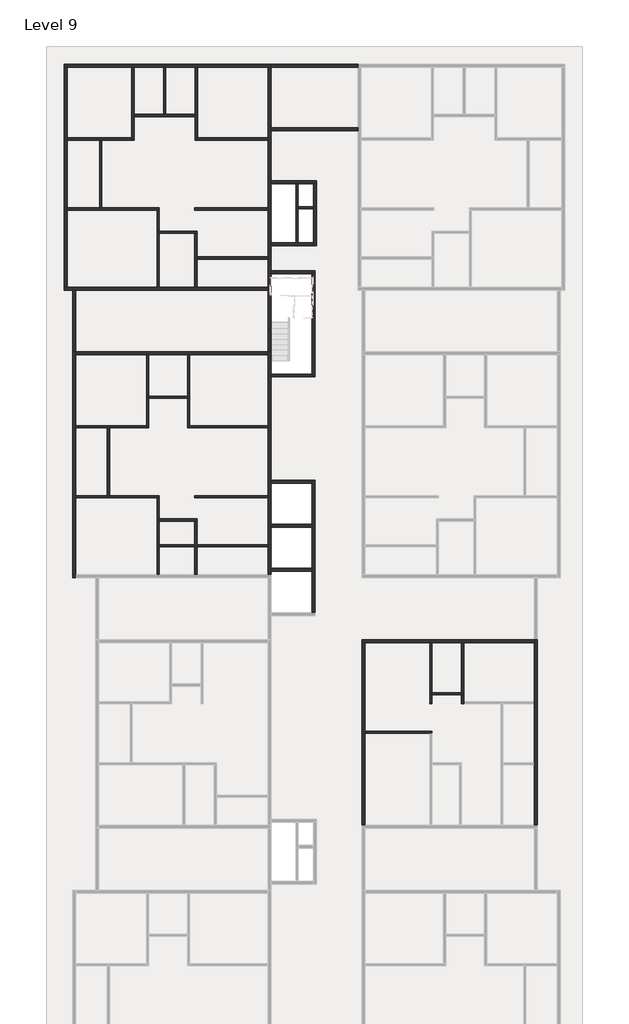
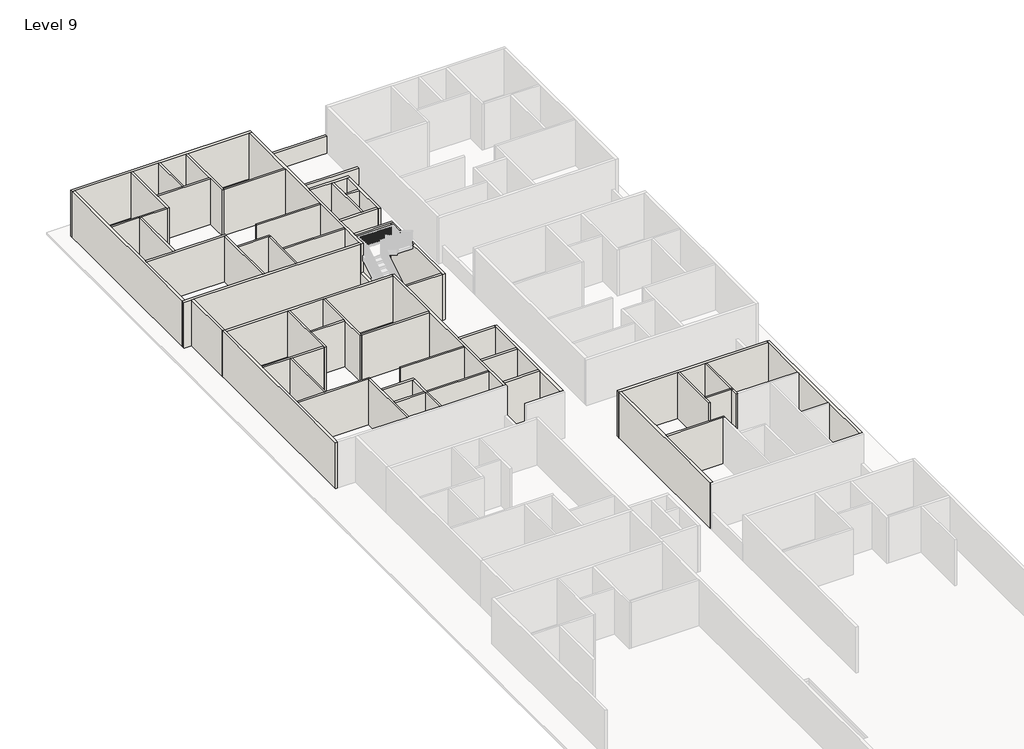
# One storey, part 3 of 8: 57 walls.
"""IFC4 building model written with IfcOpenShell, lengths in millimetres."""

from ifc_helpers import new_model, si_unit, frame, origin, place, context, project, spatial, polyline, outline, extrude, faceted_brep, element, save

model = new_model("IFC4")

# Units and contexts
model_context = context("Model", 3, world=origin())
ifc_project = project(units=[si_unit("LENGTHUNIT", "METRE", prefix="MILLI")], contexts=[model_context])

# Site, building, storey
site = spatial("IfcSite", under=ifc_project)
building = spatial("IfcBuilding", under=site)
storey = spatial("IfcBuildingStorey", under=building, Name="Level 9", Elevation=49618.6172466)

# Walls
placement = place(None, origin())
element("IfcWall", 1, ObjectType="4.5\"", at=placement, inside=storey, context=model_context, shape_type="Brep", body=[
    faceted_brep([(-10818.3415084, 35031.1216096, 49618.6172466), (-10818.3415084, 31373.5216096, 49618.6172466), (-10818.3415084, 31259.2216096, 49618.6172466), (-10818.3415084, 31259.2216096, 52666.6172466), (-10818.3415084, 31373.5216096, 52666.6172466), (-10818.3415084, 35031.1216096, 52666.6172466), (-10704.0415084, 35031.1216096, 49618.6172466), (-10704.0415084, 35031.1216096, 52666.6172466), (-10704.0415084, 32592.7216096, 52666.6172466), (-10704.0415084, 32478.4216096, 52666.6172466), (-10704.0415084, 31259.2216096, 52666.6172466), (-10704.0415084, 31259.2216096, 49618.6172466), (-10704.0415084, 32478.4216096, 49618.6172466), (-10704.0415084, 32592.7216096, 49618.6172466)], [[[0, 1, 2, 3, 4, 5]], [[6, 7, 8, 9, 10, 11, 12, 13]], [[2, 1, 0, 6, 13, 12, 11]], [[0, 5, 7, 6]], [[3, 2, 11, 10]], [[5, 4, 3, 10, 9, 8, 7]]]),
])
element("IfcWall", 2, ObjectType="4.5\"", at=placement, inside=storey, context=model_context, shape_type="Brep", body=[
    faceted_brep([(-10818.3415084, 31373.5216096, 49618.6172466), (-14171.1415084, 31373.5216096, 49618.6172466), (-14171.1415084, 31373.5216096, 52666.6172466), (-10818.3415084, 31373.5216096, 52666.6172466), (-10818.3415084, 31259.2216096, 49618.6172466), (-10818.3415084, 31259.2216096, 52666.6172466), (-12380.4415084, 31259.2216096, 52666.6172466), (-12494.7415084, 31259.2216096, 52666.6172466), (-14171.1415084, 31259.2216096, 52666.6172466), (-14171.1415084, 31259.2216096, 49618.6172466), (-12494.7415084, 31259.2216096, 49618.6172466), (-12380.4415084, 31259.2216096, 49618.6172466)], [[[0, 1, 2, 3]], [[4, 5, 6, 7, 8, 9, 10, 11]], [[1, 0, 4, 11, 10, 9]], [[0, 3, 5, 4]], [[2, 1, 9, 8]], [[3, 2, 8, 7, 6, 5]]]),
])
element("IfcWall", 3, ObjectType="4.5\"", at=placement, inside=storey, context=model_context, shape_type="SweptSolid", body=[
    extrude(outline(polyline([(-12494.7415084, 27754.0216096), (-12494.7415084, 31259.2216096), (-12380.4415084, 31259.2216096), (-12380.4415084, 27754.0216096), (-12494.7415084, 27754.0216096)])), frame((0.0, 0.0, 49618.6172466), z_axis=(0.0, 0.0, 1.0), x_axis=(1.0, 0.0, 0.0)), (0.0, 0.0, 1.0), 3048.0),
])
element("IfcWall", 4, ObjectType="4.5\"", at=placement, inside=storey, context=model_context, shape_type="Brep", body=[
    faceted_brep([(-14171.1415084, 27639.7216096, 49618.6172466), (-9510.2415084, 27639.7216096, 49618.6172466), (-9395.9415084, 27639.7216096, 49618.6172466), (-9395.9415084, 27639.7216096, 52666.6172466), (-9510.2415084, 27639.7216096, 52666.6172466), (-14171.1415084, 27639.7216096, 52666.6172466), (-14171.1415084, 27754.0216096, 49618.6172466), (-14171.1415084, 27754.0216096, 52666.6172466), (-12494.7415084, 27754.0216096, 52666.6172466), (-12380.4415084, 27754.0216096, 52666.6172466), (-9395.9415084, 27754.0216096, 52666.6172466), (-9395.9415084, 27754.0216096, 49618.6172466), (-12380.4415084, 27754.0216096, 49618.6172466), (-12494.7415084, 27754.0216096, 49618.6172466)], [[[0, 1, 2, 3, 4, 5]], [[6, 7, 8, 9, 10, 11, 12, 13]], [[2, 1, 0, 6, 13, 12, 11]], [[0, 5, 7, 6]], [[3, 2, 11, 10]], [[5, 4, 3, 10, 9, 8, 7]]]),
])
element("IfcWall", 5, ObjectType="4.5\"", at=placement, inside=storey, context=model_context, shape_type="Brep", body=[
    faceted_brep([(-9510.2415084, 27639.7216096, 49618.6172466), (-9510.2415084, 23651.9216096, 49618.6172466), (-9510.2415084, 23651.9216096, 52666.6172466), (-9510.2415084, 27639.7216096, 52666.6172466), (-9395.9415084, 27639.7216096, 49618.6172466), (-9395.9415084, 27639.7216096, 52666.6172466), (-9395.9415084, 26547.5216096, 52666.6172466), (-9395.9415084, 26433.2216096, 52666.6172466), (-9395.9415084, 23651.9216096, 52666.6172466), (-9395.9415084, 23651.9216096, 49618.6172466), (-9395.9415084, 26433.2216096, 49618.6172466), (-9395.9415084, 26547.5216096, 49618.6172466)], [[[0, 1, 2, 3]], [[4, 5, 6, 7, 8, 9, 10, 11]], [[1, 0, 4, 11, 10, 9]], [[0, 3, 5, 4]], [[2, 1, 9, 8]], [[3, 2, 8, 7, 6, 5]]]),
])
element("IfcWall", 6, ObjectType="4.5\"", at=placement, inside=storey, context=model_context, shape_type="Brep", body=[
    faceted_brep([(-9395.9415084, 26433.2216096, 49618.6172466), (-7567.1415084, 26433.2216096, 49618.6172466), (-7452.8415084, 26433.2216096, 49618.6172466), (-7452.8415084, 26433.2216096, 52666.6172466), (-7567.1415084, 26433.2216096, 52666.6172466), (-9395.9415084, 26433.2216096, 52666.6172466), (-9395.9415084, 26547.5216096, 49618.6172466), (-9395.9415084, 26547.5216096, 52666.6172466), (-7452.8415084, 26547.5216096, 52666.6172466), (-7452.8415084, 26547.5216096, 49618.6172466)], [[[0, 1, 2, 3, 4, 5]], [[6, 7, 8, 9]], [[2, 1, 0, 6, 9]], [[0, 5, 7, 6]], [[3, 2, 9, 8]], [[5, 4, 3, 8, 7]]]),
])
element("IfcWall", 7, ObjectType="4.5\"", at=placement, inside=storey, context=model_context, shape_type="Brep", body=[
    faceted_brep([(-7567.1415084, 26433.2216096, 49618.6172466), (-7567.1415084, 23651.9216096, 49618.6172466), (-7567.1415084, 23651.9216096, 52666.6172466), (-7567.1415084, 26433.2216096, 52666.6172466), (-7452.8415084, 26433.2216096, 49618.6172466), (-7452.8415084, 26433.2216096, 52666.6172466), (-7452.8415084, 25214.0216096, 52666.6172466), (-7452.8415084, 25099.7216096, 52666.6172466), (-7452.8415084, 23651.9216096, 52666.6172466), (-7452.8415084, 23651.9216096, 49618.6172466), (-7452.8415084, 25099.7216096, 49618.6172466), (-7452.8415084, 25214.0216096, 49618.6172466)], [[[0, 1, 2, 3]], [[4, 5, 6, 7, 8, 9, 10, 11]], [[1, 0, 4, 11, 10, 9]], [[0, 3, 5, 4]], [[2, 1, 9, 8]], [[3, 2, 8, 7, 6, 5]]]),
])
element("IfcWall", 8, ObjectType="4.5\"", at=placement, inside=storey, context=model_context, shape_type="SweptSolid", body=[
    extrude(outline(polyline([(-7452.8415084, 25214.0216096), (-3769.8415084, 25214.0216096), (-3769.8415084, 25099.7216096), (-7452.8415084, 25099.7216096), (-7452.8415084, 25214.0216096)])), frame((0.0, 0.0, 49618.6172466), z_axis=(0.0, 0.0, 1.0), x_axis=(1.0, 0.0, 0.0)), (0.0, 0.0, 1.0), 3048.0),
])
element("IfcWall", 9, ObjectType="4.5\"", at=placement, inside=storey, context=model_context, shape_type="SweptSolid", body=[
    extrude(outline(polyline([(-3769.8415084, 27639.7216096), (-7567.1415084, 27639.7216096), (-7567.1415084, 27754.0216096), (-3769.8415084, 27754.0216096), (-3769.8415084, 27639.7216096)])), frame((0.0, 0.0, 49618.6172466), z_axis=(0.0, 0.0, 1.0), x_axis=(1.0, 0.0, 0.0)), (0.0, 0.0, 1.0), 3048.0),
])
element("IfcWall", 10, ObjectType="4.5\"", at=placement, inside=storey, context=model_context, shape_type="Brep", body=[
    faceted_brep([(-10704.0415084, 32478.4216096, 49618.6172466), (-7541.7415084, 32478.4216096, 49618.6172466), (-7541.7415084, 32478.4216096, 52666.6172466), (-10704.0415084, 32478.4216096, 52666.6172466), (-10704.0415084, 32592.7216096, 49618.6172466), (-10704.0415084, 32592.7216096, 52666.6172466), (-9180.0415084, 32592.7216096, 52666.6172466), (-9065.7415084, 32592.7216096, 52666.6172466), (-7541.7415084, 32592.7216096, 52666.6172466), (-7541.7415084, 32592.7216096, 49618.6172466), (-9065.7415084, 32592.7216096, 49618.6172466), (-9180.0415084, 32592.7216096, 49618.6172466)], [[[0, 1, 2, 3]], [[4, 5, 6, 7, 8, 9, 10, 11]], [[1, 0, 4, 11, 10, 9]], [[0, 3, 5, 4]], [[2, 1, 9, 8]], [[3, 2, 8, 7, 6, 5]]]),
])
element("IfcWall", 11, ObjectType="4.5\"", at=placement, inside=storey, context=model_context, shape_type="SweptSolid", body=[
    extrude(outline(polyline([(-9180.0415084, 32592.7216096), (-9180.0415084, 35031.1216096), (-9065.7415084, 35031.1216096), (-9065.7415084, 32592.7216096), (-9180.0415084, 32592.7216096)])), frame((0.0, 0.0, 49618.6172466), z_axis=(0.0, 0.0, 1.0), x_axis=(1.0, 0.0, 0.0)), (0.0, 0.0, 1.0), 3048.0),
])
element("IfcWall", 12, ObjectType="4.5\"", at=placement, inside=storey, context=model_context, shape_type="Brep", body=[
    faceted_brep([(-7541.7415084, 35031.1216096, 49618.6172466), (-7541.7415084, 32592.7216096, 49618.6172466), (-7541.7415084, 32478.4216096, 49618.6172466), (-7541.7415084, 31259.2216096, 49618.6172466), (-7541.7415084, 31259.2216096, 52666.6172466), (-7541.7415084, 32478.4216096, 52666.6172466), (-7541.7415084, 32592.7216096, 52666.6172466), (-7541.7415084, 35031.1216096, 52666.6172466), (-7427.4415084, 35031.1216096, 49618.6172466), (-7427.4415084, 35031.1216096, 52666.6172466), (-7427.4415084, 31373.5216096, 52666.6172466), (-7427.4415084, 31259.2216096, 52666.6172466), (-7427.4415084, 31259.2216096, 49618.6172466), (-7427.4415084, 31373.5216096, 49618.6172466)], [[[0, 1, 2, 3, 4, 5, 6, 7]], [[8, 9, 10, 11, 12, 13]], [[3, 2, 1, 0, 8, 13, 12]], [[0, 7, 9, 8]], [[4, 3, 12, 11]], [[7, 6, 5, 4, 11, 10, 9]]]),
])
element("IfcWall", 13, ObjectType="4.5\"", at=placement, inside=storey, context=model_context, shape_type="SweptSolid", body=[
    extrude(outline(polyline([(-3769.8415084, 31259.2216096), (-7427.4415084, 31259.2216096), (-7427.4415084, 31373.5216096), (-3769.8415084, 31373.5216096), (-3769.8415084, 31259.2216096)])), frame((0.0, 0.0, 49618.6172466), z_axis=(0.0, 0.0, 1.0), x_axis=(1.0, 0.0, 0.0)), (0.0, 0.0, 1.0), 3048.0),
])
element("IfcWall", 14, ObjectType="4.5\"", at=placement, inside=storey, context=model_context, shape_type="Brep", body=[
    faceted_brep([(-10061.4044854, 20146.7216096, 49618.6172466), (-10061.4044854, 16489.1216096, 49618.6172466), (-10061.4044854, 16374.8216096, 49618.6172466), (-10061.4044854, 16374.8216096, 52666.6172466), (-10061.4044854, 16489.1216096, 52666.6172466), (-10061.4044854, 20146.7216096, 52666.6172466), (-9947.1044854, 20146.7216096, 49618.6172466), (-9947.1044854, 20146.7216096, 52666.6172466), (-9947.1044854, 18013.1216096, 52666.6172466), (-9947.1044854, 17898.8216096, 52666.6172466), (-9947.1044854, 16374.8216096, 52666.6172466), (-9947.1044854, 16374.8216096, 49618.6172466), (-9947.1044854, 17898.8216096, 49618.6172466), (-9947.1044854, 18013.1216096, 49618.6172466)], [[[0, 1, 2, 3, 4, 5]], [[6, 7, 8, 9, 10, 11, 12, 13]], [[2, 1, 0, 6, 13, 12, 11]], [[0, 5, 7, 6]], [[3, 2, 11, 10]], [[5, 4, 3, 10, 9, 8, 7]]]),
])
element("IfcWall", 15, ObjectType="4.5\"", at=placement, inside=storey, context=model_context, shape_type="Brep", body=[
    faceted_brep([(-10061.4044854, 16489.1216096, 49618.6172466), (-13719.0044854, 16489.1216096, 49618.6172466), (-13719.0044854, 16489.1216096, 52666.6172466), (-10061.4044854, 16489.1216096, 52666.6172466), (-10061.4044854, 16374.8216096, 49618.6172466), (-10061.4044854, 16374.8216096, 52666.6172466), (-11980.3915084, 16374.8216096, 52666.6172466), (-12094.6915084, 16374.8216096, 52666.6172466), (-13719.0044854, 16374.8216096, 52666.6172466), (-13719.0044854, 16374.8216096, 49618.6172466), (-12094.6915084, 16374.8216096, 49618.6172466), (-11980.3915084, 16374.8216096, 49618.6172466)], [[[0, 1, 2, 3]], [[4, 5, 6, 7, 8, 9, 10, 11]], [[1, 0, 4, 11, 10, 9]], [[0, 3, 5, 4]], [[2, 1, 9, 8]], [[3, 2, 8, 7, 6, 5]]]),
])
element("IfcWall", 16, ObjectType="4.5\"", at=placement, inside=storey, context=model_context, shape_type="SweptSolid", body=[
    extrude(outline(polyline([(-7940.5044854, 17898.8216096), (-9947.1044854, 17898.8216096), (-9947.1044854, 18013.1216096), (-7940.5044854, 18013.1216096), (-7940.5044854, 17898.8216096)])), frame((0.0, 0.0, 49618.6172466), z_axis=(0.0, 0.0, 1.0), x_axis=(1.0, 0.0, 0.0)), (0.0, 0.0, 1.0), 3048.0),
])
element("IfcWall", 17, ObjectType="4.5\"", at=placement, inside=storey, context=model_context, shape_type="Brep", body=[
    faceted_brep([(-7940.5044854, 20146.7216096, 49618.6172466), (-7940.5044854, 18013.1216096, 49618.6172466), (-7940.5044854, 17898.8216096, 49618.6172466), (-7940.5044854, 16374.8216096, 49618.6172466), (-7940.5044854, 16374.8216096, 52666.6172466), (-7940.5044854, 17898.8216096, 52666.6172466), (-7940.5044854, 18013.1216096, 52666.6172466), (-7940.5044854, 20146.7216096, 52666.6172466), (-7826.2044854, 20146.7216096, 49618.6172466), (-7826.2044854, 20146.7216096, 52666.6172466), (-7826.2044854, 16489.1216096, 52666.6172466), (-7826.2044854, 16374.8216096, 52666.6172466), (-7826.2044854, 16374.8216096, 49618.6172466), (-7826.2044854, 16489.1216096, 49618.6172466)], [[[0, 1, 2, 3, 4, 5, 6, 7]], [[8, 9, 10, 11, 12, 13]], [[3, 2, 1, 0, 8, 13, 12]], [[0, 7, 9, 8]], [[4, 3, 12, 11]], [[7, 6, 5, 4, 11, 10, 9]]]),
])
element("IfcWall", 18, ObjectType="4.5\"", at=placement, inside=storey, context=model_context, shape_type="SweptSolid", body=[
    extrude(outline(polyline([(-3769.8415084, 16374.8216096), (-7826.2044854, 16374.8216096), (-7826.2044854, 16489.1216096), (-3769.8415084, 16489.1216096), (-3769.8415084, 16374.8216096)])), frame((0.0, 0.0, 49618.6172466), z_axis=(0.0, 0.0, 1.0), x_axis=(1.0, 0.0, 0.0)), (0.0, 0.0, 1.0), 3048.0),
])
element("IfcWall", 19, ObjectType="4.5\"", at=placement, inside=storey, context=model_context, shape_type="SweptSolid", body=[
    extrude(outline(polyline([(-12094.6915084, 12869.6216096), (-12094.6915084, 16374.8216096), (-11980.3915084, 16374.8216096), (-11980.3915084, 12869.6216096), (-12094.6915084, 12869.6216096)])), frame((0.0, 0.0, 49618.6172466), z_axis=(0.0, 0.0, 1.0), x_axis=(1.0, 0.0, 0.0)), (0.0, 0.0, 1.0), 3048.0),
])
element("IfcWall", 20, ObjectType="4.5\"", at=placement, inside=storey, context=model_context, shape_type="Brep", body=[
    faceted_brep([(-13719.0044854, 12755.3216096, 49618.6172466), (-9510.2415084, 12755.3216096, 49618.6172466), (-9395.9415084, 12755.3216096, 49618.6172466), (-9395.9415084, 12755.3216096, 52666.6172466), (-9510.2415084, 12755.3216096, 52666.6172466), (-13719.0044854, 12755.3216096, 52666.6172466), (-13719.0044854, 12869.6216096, 49618.6172466), (-13719.0044854, 12869.6216096, 52666.6172466), (-12094.6915084, 12869.6216096, 52666.6172466), (-11980.3915084, 12869.6216096, 52666.6172466), (-9395.9415084, 12869.6216096, 52666.6172466), (-9395.9415084, 12869.6216096, 49618.6172466), (-11980.3915084, 12869.6216096, 49618.6172466), (-12094.6915084, 12869.6216096, 49618.6172466)], [[[0, 1, 2, 3, 4, 5]], [[6, 7, 8, 9, 10, 11, 12, 13]], [[2, 1, 0, 6, 13, 12, 11]], [[0, 5, 7, 6]], [[3, 2, 11, 10]], [[5, 4, 3, 10, 9, 8, 7]]]),
])
element("IfcWall", 21, ObjectType="4.5\"", at=placement, inside=storey, context=model_context, shape_type="Brep", body=[
    faceted_brep([(-9510.2415084, 12755.3216096, 49618.6172466), (-9510.2415084, 8767.5216096, 49618.6172466), (-9510.2415084, 8767.5216096, 52666.6172466), (-9510.2415084, 12755.3216096, 52666.6172466), (-9395.9415084, 12755.3216096, 49618.6172466), (-9395.9415084, 12755.3216096, 52666.6172466), (-9395.9415084, 11663.1216096, 52666.6172466), (-9395.9415084, 11548.8216096, 52666.6172466), (-9395.9415084, 10329.6216096, 52666.6172466), (-9395.9415084, 10215.3216096, 52666.6172466), (-9395.9415084, 8767.5216096, 52666.6172466), (-9395.9415084, 8767.5216096, 49618.6172466), (-9395.9415084, 10215.3216096, 49618.6172466), (-9395.9415084, 10329.6216096, 49618.6172466), (-9395.9415084, 11548.8216096, 49618.6172466), (-9395.9415084, 11663.1216096, 49618.6172466)], [[[0, 1, 2, 3]], [[4, 5, 6, 7, 8, 9, 10, 11, 12, 13, 14, 15]], [[1, 0, 4, 15, 14, 13, 12, 11]], [[0, 3, 5, 4]], [[2, 1, 11, 10]], [[3, 2, 10, 9, 8, 7, 6, 5]]]),
])
element("IfcWall", 22, ObjectType="4.5\"", at=placement, inside=storey, context=model_context, shape_type="SweptSolid", body=[
    extrude(outline(polyline([(-7567.1415084, 10215.3216096), (-9395.9415084, 10215.3216096), (-9395.9415084, 10329.6216096), (-7567.1415084, 10329.6216096), (-7567.1415084, 10215.3216096)])), frame((0.0, 0.0, 49618.6172466), z_axis=(0.0, 0.0, 1.0), x_axis=(1.0, 0.0, 0.0)), (0.0, 0.0, 1.0), 3048.0),
])
element("IfcWall", 23, ObjectType="4.5\"", at=placement, inside=storey, context=model_context, shape_type="Brep", body=[
    faceted_brep([(-9395.9415084, 11548.8216096, 49618.6172466), (-7567.1415084, 11548.8216096, 49618.6172466), (-7452.8415084, 11548.8216096, 49618.6172466), (-7452.8415084, 11548.8216096, 52666.6172466), (-7567.1415084, 11548.8216096, 52666.6172466), (-9395.9415084, 11548.8216096, 52666.6172466), (-9395.9415084, 11663.1216096, 49618.6172466), (-9395.9415084, 11663.1216096, 52666.6172466), (-7452.8415084, 11663.1216096, 52666.6172466), (-7452.8415084, 11663.1216096, 49618.6172466)], [[[0, 1, 2, 3, 4, 5]], [[6, 7, 8, 9]], [[2, 1, 0, 6, 9]], [[0, 5, 7, 6]], [[3, 2, 9, 8]], [[5, 4, 3, 8, 7]]]),
])
element("IfcWall", 24, ObjectType="4.5\"", at=placement, inside=storey, context=model_context, shape_type="Brep", body=[
    faceted_brep([(-7567.1415084, 11548.8216096, 49618.6172466), (-7567.1415084, 10329.6216096, 49618.6172466), (-7567.1415084, 10215.3216096, 49618.6172466), (-7567.1415084, 8767.5216096, 49618.6172466), (-7567.1415084, 8767.5216096, 52666.6172466), (-7567.1415084, 10215.3216096, 52666.6172466), (-7567.1415084, 10329.6216096, 52666.6172466), (-7567.1415084, 11548.8216096, 52666.6172466), (-7452.8415084, 11548.8216096, 49618.6172466), (-7452.8415084, 11548.8216096, 52666.6172466), (-7452.8415084, 10329.6216096, 52666.6172466), (-7452.8415084, 10215.3216096, 52666.6172466), (-7452.8415084, 8767.5216096, 52666.6172466), (-7452.8415084, 8767.5216096, 49618.6172466), (-7452.8415084, 10215.3216096, 49618.6172466), (-7452.8415084, 10329.6216096, 49618.6172466)], [[[0, 1, 2, 3, 4, 5, 6, 7]], [[8, 9, 10, 11, 12, 13, 14, 15]], [[3, 2, 1, 0, 8, 15, 14, 13]], [[0, 7, 9, 8]], [[4, 3, 13, 12]], [[7, 6, 5, 4, 12, 11, 10, 9]]]),
])
element("IfcWall", 25, ObjectType="4.5\"", at=placement, inside=storey, context=model_context, shape_type="SweptSolid", body=[
    extrude(outline(polyline([(-3769.8415084, 10215.3216096), (-7452.8415084, 10215.3216096), (-7452.8415084, 10329.6216096), (-3769.8415084, 10329.6216096), (-3769.8415084, 10215.3216096)])), frame((0.0, 0.0, 49618.6172466), z_axis=(0.0, 0.0, 1.0), x_axis=(1.0, 0.0, 0.0)), (0.0, 0.0, 1.0), 3048.0),
])
element("IfcWall", 26, ObjectType="4.5\"", at=placement, inside=storey, context=model_context, shape_type="SweptSolid", body=[
    extrude(outline(polyline([(-3769.8415084, 12755.3216096), (-7567.1415084, 12755.3216096), (-7567.1415084, 12869.6216096), (-3769.8415084, 12869.6216096), (-3769.8415084, 12755.3216096)])), frame((0.0, 0.0, 49618.6172466), z_axis=(0.0, 0.0, 1.0), x_axis=(1.0, 0.0, 0.0)), (0.0, 0.0, 1.0), 3048.0),
])
element("IfcWall", 27, ObjectType="4.5\"", at=placement, inside=storey, context=model_context, shape_type="Brep", body=[
    faceted_brep([(1259.3584916, 572.7745083, 49618.6172466), (4610.8714687, 572.7745083, 49618.6172466), (4725.1714687, 572.7745083, 49618.6172466), (4725.1714687, 572.7745083, 52666.6172466), (4610.8714687, 572.7745083, 52666.6172466), (1259.3584916, 572.7745083, 52666.6172466), (1259.3584916, 687.0745083, 49618.6172466), (1259.3584916, 687.0745083, 52666.6172466), (4725.1714687, 687.0745083, 52666.6172466), (4725.1714687, 687.0745083, 49618.6172466)], [[[0, 1, 2, 3, 4, 5]], [[6, 7, 8, 9]], [[2, 1, 0, 6, 9]], [[0, 5, 7, 6]], [[3, 2, 9, 8]], [[5, 4, 3, 8, 7]]]),
])
element("IfcWall", 28, ObjectType="4.5\"", at=placement, inside=storey, context=model_context, shape_type="Brep", body=[
    faceted_brep([(4610.8714687, 5262.3216096, 49618.6172466), (4610.8714687, 2100.0216096, 49618.6172466), (4610.8714687, 2100.0216096, 52666.6172466), (4610.8714687, 5262.3216096, 52666.6172466), (4725.1714687, 5262.3216096, 49618.6172466), (4725.1714687, 5262.3216096, 52666.6172466), (4725.1714687, 2671.5216096, 52666.6172466), (4725.1714687, 2557.2216096, 52666.6172466), (4725.1714687, 2100.0216096, 52666.6172466), (4725.1714687, 2100.0216096, 49618.6172466), (4725.1714687, 2557.2216096, 49618.6172466), (4725.1714687, 2671.5216096, 49618.6172466)], [[[0, 1, 2, 3]], [[4, 5, 6, 7, 8, 9, 10, 11]], [[1, 0, 4, 11, 10, 9]], [[2, 1, 9, 8]], [[0, 3, 5, 4]], [[3, 2, 8, 7, 6, 5]]]),
])
element("IfcWall", 29, ObjectType="4.5\"", at=placement, inside=storey, context=model_context, shape_type="Brep", body=[
    faceted_brep([(4725.1714687, 2557.2216096, 49618.6172466), (6249.1714687, 2557.2216096, 49618.6172466), (6363.4714687, 2557.2216096, 49618.6172466), (6363.4714687, 2557.2216096, 52666.6172466), (6249.1714687, 2557.2216096, 52666.6172466), (4725.1714687, 2557.2216096, 52666.6172466), (4725.1714687, 2671.5216096, 49618.6172466), (4725.1714687, 2671.5216096, 52666.6172466), (6249.1714687, 2671.5216096, 52666.6172466), (6363.4714687, 2671.5216096, 52666.6172466), (6363.4714687, 2671.5216096, 49618.6172466), (6249.1714687, 2671.5216096, 49618.6172466)], [[[0, 1, 2, 3, 4, 5]], [[6, 7, 8, 9, 10, 11]], [[2, 1, 0, 6, 11, 10]], [[0, 5, 7, 6]], [[3, 2, 10, 9]], [[5, 4, 3, 9, 8, 7]]]),
])
element("IfcWall", 30, ObjectType="4.5\"", at=placement, inside=storey, context=model_context, shape_type="SweptSolid", body=[
    extrude(outline(polyline([(6363.4714687, 5262.3216096), (6363.4714687, 2671.5216096), (6249.1714687, 2671.5216096), (6249.1714687, 5262.3216096), (6363.4714687, 5262.3216096)])), frame((0.0, 0.0, 49618.6172466), z_axis=(0.0, 0.0, 1.0), x_axis=(1.0, 0.0, 0.0)), (0.0, 0.0, 1.0), 3048.0),
])
element("IfcWall", 31, ObjectType="4.5\"", at=placement, inside=storey, context=model_context, shape_type="Brep", body=[
    faceted_brep([(6249.1714687, 2557.2216096, 49618.6172466), (6249.1714687, 2100.0216096, 49618.6172466), (6249.1714687, 2100.0216096, 52666.6172466), (6249.1714687, 2557.2216096, 52666.6172466), (6363.4714687, 2557.2216096, 49618.6172466), (6363.4714687, 2557.2216096, 52666.6172466), (6363.4714687, 2214.3216096, 52666.6172466), (6363.4714687, 2100.0216096, 52666.6172466), (6363.4714687, 2100.0216096, 49618.6172466), (6363.4714687, 2214.3216096, 49618.6172466)], [[[0, 1, 2, 3]], [[4, 5, 6, 7, 8, 9]], [[1, 0, 4, 9, 8]], [[0, 3, 5, 4]], [[2, 1, 8, 7]], [[3, 2, 7, 6, 5]]]),
])
element("IfcWall", 32, ObjectType="4.5\"", at=placement, inside=storey, context=model_context, shape_type="Brep", body=[
    faceted_brep([(-2321.9738684, 29000.0900967, 49618.6172466), (-2321.9738684, 25952.0900967, 49618.6172466), (-2321.9738684, 25952.0900967, 52666.6172466), (-2321.9738684, 29000.0900967, 52666.6172466), (-2207.6738684, 29000.0900967, 49618.6172466), (-2207.6738684, 29000.0900967, 52666.6172466), (-2207.6738684, 27820.8172885, 52666.6172466), (-2207.6738684, 27706.5172885, 52666.6172466), (-2207.6738684, 25952.0900967, 52666.6172466), (-2207.6738684, 25952.0900967, 49618.6172466), (-2207.6738684, 27706.5172885, 49618.6172466), (-2207.6738684, 27820.8172885, 49618.6172466)], [[[0, 1, 2, 3]], [[4, 5, 6, 7, 8, 9, 10, 11]], [[1, 0, 4, 11, 10, 9]], [[3, 2, 8, 7, 6, 5]], [[0, 3, 5, 4]], [[2, 1, 9, 8]]]),
])
element("IfcWall", 33, ObjectType="4.5\"", at=placement, inside=storey, context=model_context, shape_type="SweptSolid", body=[
    extrude(outline(polyline([(-2207.6738684, 27820.8172885), (-1407.6415084, 27820.8172885), (-1407.6415084, 27706.5172885), (-2207.6738684, 27706.5172885), (-2207.6738684, 27820.8172885)])), frame((0.0, 0.0, 49618.6172466), z_axis=(0.0, 0.0, 1.0), x_axis=(1.0, 0.0, 0.0)), (0.0, 0.0, 1.0), 3048.0),
])
element("IfcWall", 34, ObjectType="6\"", at=placement, inside=storey, context=model_context, shape_type="Brep", body=[
    faceted_brep([(-14323.5415084, 35031.1216096, 49618.6172466), (-14171.1415084, 35031.1216096, 49618.6172466), (-10818.3415084, 35031.1216096, 49618.6172466), (-10704.0415084, 35031.1216096, 49618.6172466), (-9180.0415084, 35031.1216096, 49618.6172466), (-9065.7415084, 35031.1216096, 49618.6172466), (-7541.7415084, 35031.1216096, 49618.6172466), (-7427.4415084, 35031.1216096, 49618.6172466), (-3769.8415084, 35031.1216096, 49618.6172466), (-3617.4415084, 35031.1216096, 49618.6172466), (-3617.4415084, 35031.1216096, 52666.6172466), (-3769.8415084, 35031.1216096, 52666.6172466), (-7427.4415084, 35031.1216096, 52666.6172466), (-7541.7415084, 35031.1216096, 52666.6172466), (-9065.7415084, 35031.1216096, 52666.6172466), (-9180.0415084, 35031.1216096, 52666.6172466), (-10704.0415084, 35031.1216096, 52666.6172466), (-10818.3415084, 35031.1216096, 52666.6172466), (-14171.1415084, 35031.1216096, 52666.6172466), (-14323.5415084, 35031.1216096, 52666.6172466), (-14323.5415084, 35183.5216096, 49618.6172466), (-14323.5415084, 35183.5216096, 52666.6172466), (-3617.4415084, 35183.5216096, 52666.6172466), (-3617.4415084, 35183.5216096, 49618.6172466)], [[[0, 1, 2, 3, 4, 5, 6, 7, 8, 9, 10, 11, 12, 13, 14, 15, 16, 17, 18, 19]], [[20, 21, 22, 23]], [[9, 8, 7, 6, 5, 4, 3, 2, 1, 0, 20, 23]], [[0, 19, 21, 20]], [[9, 23, 22, 10]], [[19, 18, 17, 16, 15, 14, 13, 12, 11, 10, 22, 21]]]),
])
element("IfcWall", 35, ObjectType="6\"", at=placement, inside=storey, context=model_context, shape_type="Brep", body=[
    faceted_brep([(-3769.8415084, 35031.1216096, 52666.6172466), (-3769.8415084, 35031.1216096, 49618.6172466), (-3769.8415084, 31373.5216096, 49618.6172466), (-3769.8415084, 31259.2216096, 49618.6172466), (-3769.8415084, 27754.0216096, 49618.6172466), (-3769.8415084, 27639.7216096, 49618.6172466), (-3769.8415084, 25214.0216096, 49618.6172466), (-3769.8415084, 25099.7216096, 49618.6172466), (-3769.8415084, 23651.9216096, 49618.6172466), (-3769.8415084, 23499.5216096, 49618.6172466), (-3769.8415084, 23499.5216096, 52666.6172466), (-3769.8415084, 23651.9216096, 52666.6172466), (-3769.8415084, 25099.7216096, 52666.6172466), (-3769.8415084, 25214.0216096, 52666.6172466), (-3769.8415084, 27639.7216096, 52666.6172466), (-3769.8415084, 27754.0216096, 52666.6172466), (-3769.8415084, 31259.2216096, 52666.6172466), (-3769.8415084, 31373.5216096, 52666.6172466), (-3617.4415084, 35031.1216096, 49618.6172466), (-3617.4415084, 35031.1216096, 52666.6172466), (-3617.4415084, 29152.4900967, 52666.6172466), (-3617.4415084, 29000.0900967, 52666.6172466), (-3617.4415084, 25952.0900967, 52666.6172466), (-3617.4415084, 25799.6900967, 52666.6172466), (-3617.4415084, 24490.1216096, 52666.6172466), (-3617.4415084, 24337.7216096, 52666.6172466), (-3617.4415084, 23499.5216096, 52666.6172466), (-3617.4415084, 23499.5216096, 49618.6172466), (-3617.4415084, 24337.7216096, 49618.6172466), (-3617.4415084, 24490.1216096, 49618.6172466), (-3617.4415084, 25799.6900967, 49618.6172466), (-3617.4415084, 25952.0900967, 49618.6172466), (-3617.4415084, 29000.0900967, 49618.6172466), (-3617.4415084, 29152.4900967, 49618.6172466), (-3617.4415084, 31744.9197155, 49618.6172466), (-3617.4415084, 31897.3197155, 49618.6172466)], [[[0, 1, 2, 3, 4, 5, 6, 7, 8, 9, 10, 11, 12, 13, 14, 15, 16, 17]], [[18, 19, 20, 21, 22, 23, 24, 25, 26, 27, 28, 29, 30, 31, 32, 33, 34, 35]], [[9, 8, 7, 6, 5, 4, 3, 2, 1, 18, 35, 34, 33, 32, 31, 30, 29, 28, 27]], [[0, 19, 18, 1]], [[9, 27, 26, 10]], [[0, 17, 16, 15, 14, 13, 12, 11, 10, 26, 25, 24, 23, 22, 21, 20, 19]]]),
])
element("IfcWall", 36, ObjectType="6\"", at=placement, inside=storey, context=model_context, shape_type="Brep", body=[
    faceted_brep([(-3769.8415084, 23651.9216096, 52666.6172466), (-3769.8415084, 23651.9216096, 49618.6172466), (-7452.8415084, 23651.9216096, 49618.6172466), (-7567.1415084, 23651.9216096, 49618.6172466), (-9395.9415084, 23651.9216096, 49618.6172466), (-9510.2415084, 23651.9216096, 49618.6172466), (-14171.1415084, 23651.9216096, 49618.6172466), (-14323.5415084, 23651.9216096, 49618.6172466), (-14323.5415084, 23651.9216096, 52666.6172466), (-14171.1415084, 23651.9216096, 52666.6172466), (-9510.2415084, 23651.9216096, 52666.6172466), (-9395.9415084, 23651.9216096, 52666.6172466), (-7567.1415084, 23651.9216096, 52666.6172466), (-7452.8415084, 23651.9216096, 52666.6172466), (-3769.8415084, 23499.5216096, 49618.6172466), (-3769.8415084, 23499.5216096, 52666.6172466), (-13719.0044854, 23499.5216096, 52666.6172466), (-13871.4044854, 23499.5216096, 52666.6172466), (-14323.5415084, 23499.5216096, 52666.6172466), (-14323.5415084, 23499.5216096, 49618.6172466), (-13871.4044854, 23499.5216096, 49618.6172466), (-13719.0044854, 23499.5216096, 49618.6172466)], [[[0, 1, 2, 3, 4, 5, 6, 7, 8, 9, 10, 11, 12, 13]], [[14, 15, 16, 17, 18, 19, 20, 21]], [[7, 6, 5, 4, 3, 2, 1, 14, 21, 20, 19]], [[8, 7, 19, 18]], [[0, 15, 14, 1]], [[0, 13, 12, 11, 10, 9, 8, 18, 17, 16, 15]]]),
])
element("IfcWall", 37, ObjectType="6\"", at=placement, inside=storey, context=model_context, shape_type="Brep", body=[
    faceted_brep([(-14171.1415084, 23651.9216096, 49618.6172466), (-14171.1415084, 27639.7216096, 49618.6172466), (-14171.1415084, 27754.0216096, 49618.6172466), (-14171.1415084, 31259.2216096, 49618.6172466), (-14171.1415084, 31373.5216096, 49618.6172466), (-14171.1415084, 35031.1216096, 49618.6172466), (-14171.1415084, 35031.1216096, 52666.6172466), (-14171.1415084, 31373.5216096, 52666.6172466), (-14171.1415084, 31259.2216096, 52666.6172466), (-14171.1415084, 27754.0216096, 52666.6172466), (-14171.1415084, 27639.7216096, 52666.6172466), (-14171.1415084, 23651.9216096, 52666.6172466), (-14323.5415084, 23651.9216096, 49618.6172466), (-14323.5415084, 23651.9216096, 52666.6172466), (-14323.5415084, 35031.1216096, 52666.6172466), (-14323.5415084, 35031.1216096, 49618.6172466)], [[[0, 1, 2, 3, 4, 5, 6, 7, 8, 9, 10, 11]], [[12, 13, 14, 15]], [[5, 4, 3, 2, 1, 0, 12, 15]], [[6, 5, 15, 14]], [[0, 11, 13, 12]], [[11, 10, 9, 8, 7, 6, 14, 13]]]),
])
element("IfcWall", 38, ObjectType="6\"", at=placement, inside=storey, context=model_context, shape_type="Brep", body=[
    faceted_brep([(-13871.4044854, 20299.1216096, 49618.6172466), (-13871.4044854, 8615.1216096, 49618.6172466), (-13871.4044854, 8615.1216096, 52666.6172466), (-13871.4044854, 20299.1216096, 52666.6172466), (-13719.0044854, 20299.1216096, 49618.6172466), (-13719.0044854, 20299.1216096, 52666.6172466), (-13719.0044854, 20146.7216096, 52666.6172466), (-13719.0044854, 16489.1216096, 52666.6172466), (-13719.0044854, 16374.8216096, 52666.6172466), (-13719.0044854, 12869.6216096, 52666.6172466), (-13719.0044854, 12755.3216096, 52666.6172466), (-13719.0044854, 8767.5216096, 52666.6172466), (-13719.0044854, 8615.1216096, 52666.6172466), (-13719.0044854, 8615.1216096, 49618.6172466), (-13719.0044854, 8767.5216096, 49618.6172466), (-13719.0044854, 12755.3216096, 49618.6172466), (-13719.0044854, 12869.6216096, 49618.6172466), (-13719.0044854, 16374.8216096, 49618.6172466), (-13719.0044854, 16489.1216096, 49618.6172466), (-13719.0044854, 20146.7216096, 49618.6172466)], [[[0, 1, 2, 3]], [[4, 5, 6, 7, 8, 9, 10, 11, 12, 13, 14, 15, 16, 17, 18, 19]], [[1, 0, 4, 19, 18, 17, 16, 15, 14, 13]], [[2, 1, 13, 12]], [[0, 3, 5, 4]], [[3, 2, 12, 11, 10, 9, 8, 7, 6, 5]]]),
])
element("IfcWall", 39, ObjectType="6\"", at=placement, inside=storey, context=model_context, shape_type="Brep", body=[
    faceted_brep([(-3617.4415084, 8767.5216096, 52666.6172466), (-3617.4415084, 8767.5216096, 49618.6172466), (-3617.4415084, 8945.2303368, 49618.6172466), (-3617.4415084, 9097.6303368, 49618.6172466), (-3617.4415084, 11231.2303368, 49618.6172466), (-3617.4415084, 11383.6303368, 49618.6172466), (-3617.4415084, 13517.2303368, 49618.6172466), (-3617.4415084, 13669.6303368, 49618.6172466), (-3617.4415084, 19003.7216096, 49618.6172466), (-3617.4415084, 19156.1216096, 49618.6172466), (-3617.4415084, 20299.1216096, 49618.6172466), (-3617.4415084, 20299.1216096, 52666.6172466), (-3617.4415084, 19156.1216096, 52666.6172466), (-3617.4415084, 19003.7216096, 52666.6172466), (-3617.4415084, 13669.6303368, 52666.6172466), (-3617.4415084, 13517.2303368, 52666.6172466), (-3617.4415084, 11383.6303368, 52666.6172466), (-3617.4415084, 11231.2303368, 52666.6172466), (-3617.4415084, 9097.6303368, 52666.6172466), (-3617.4415084, 8945.2303368, 52666.6172466), (-3769.8415084, 8767.5216096, 49618.6172466), (-3769.8415084, 8767.5216096, 52666.6172466), (-3769.8415084, 10215.3216096, 52666.6172466), (-3769.8415084, 10329.6216096, 52666.6172466), (-3769.8415084, 12755.3216096, 52666.6172466), (-3769.8415084, 12869.6216096, 52666.6172466), (-3769.8415084, 16374.8216096, 52666.6172466), (-3769.8415084, 16489.1216096, 52666.6172466), (-3769.8415084, 20146.7216096, 52666.6172466), (-3769.8415084, 20299.1216096, 52666.6172466), (-3769.8415084, 20299.1216096, 49618.6172466), (-3769.8415084, 20146.7216096, 49618.6172466), (-3769.8415084, 16489.1216096, 49618.6172466), (-3769.8415084, 16374.8216096, 49618.6172466), (-3769.8415084, 12869.6216096, 49618.6172466), (-3769.8415084, 12755.3216096, 49618.6172466), (-3769.8415084, 10329.6216096, 49618.6172466), (-3769.8415084, 10215.3216096, 49618.6172466)], [[[0, 1, 2, 3, 4, 5, 6, 7, 8, 9, 10, 11, 12, 13, 14, 15, 16, 17, 18, 19]], [[20, 21, 22, 23, 24, 25, 26, 27, 28, 29, 30, 31, 32, 33, 34, 35, 36, 37]], [[10, 9, 8, 7, 6, 5, 4, 3, 2, 1, 20, 37, 36, 35, 34, 33, 32, 31, 30]], [[10, 30, 29, 11]], [[0, 21, 20, 1]], [[0, 19, 18, 17, 16, 15, 14, 13, 12, 11, 29, 28, 27, 26, 25, 24, 23, 22, 21]]]),
])
element("IfcWall", 40, ObjectType="6\"", at=placement, inside=storey, context=model_context, shape_type="Brep", body=[
    faceted_brep([(-3769.8415084, 20299.1216096, 52666.6172466), (-3769.8415084, 20299.1216096, 49618.6172466), (-13719.0044854, 20299.1216096, 49618.6172466), (-13719.0044854, 20299.1216096, 52666.6172466), (-3769.8415084, 20146.7216096, 49618.6172466), (-3769.8415084, 20146.7216096, 52666.6172466), (-7826.2044854, 20146.7216096, 52666.6172466), (-7940.5044854, 20146.7216096, 52666.6172466), (-9947.1044854, 20146.7216096, 52666.6172466), (-10061.4044854, 20146.7216096, 52666.6172466), (-13719.0044854, 20146.7216096, 52666.6172466), (-13719.0044854, 20146.7216096, 49618.6172466), (-10061.4044854, 20146.7216096, 49618.6172466), (-9947.1044854, 20146.7216096, 49618.6172466), (-7940.5044854, 20146.7216096, 49618.6172466), (-7826.2044854, 20146.7216096, 49618.6172466)], [[[0, 1, 2, 3]], [[4, 5, 6, 7, 8, 9, 10, 11, 12, 13, 14, 15]], [[2, 1, 4, 15, 14, 13, 12, 11]], [[3, 2, 11, 10]], [[0, 5, 4, 1]], [[0, 3, 10, 9, 8, 7, 6, 5]]]),
])
element("IfcWall", 41, ObjectType="6\"", at=placement, inside=storey, context=model_context, shape_type="Brep", body=[
    faceted_brep([(10173.4714687, -4185.9344126, 52666.6172466), (10173.4714687, -4185.9344126, 49618.6172466), (10173.4714687, 5414.7216096, 49618.6172466), (10173.4714687, 5414.7216096, 52666.6172466), (10021.0714687, -4185.9344126, 49618.6172466), (10021.0714687, -4185.9344126, 52666.6172466), (10021.0714687, -1061.7344126, 52666.6172466), (10021.0714687, -947.4344126, 52666.6172466), (10021.0714687, 2100.0216096, 52666.6172466), (10021.0714687, 2214.3216096, 52666.6172466), (10021.0714687, 5262.3216096, 52666.6172466), (10021.0714687, 5414.7216096, 52666.6172466), (10021.0714687, 5414.7216096, 49618.6172466), (10021.0714687, 5262.3216096, 49618.6172466), (10021.0714687, 2214.3216096, 49618.6172466), (10021.0714687, 2100.0216096, 49618.6172466), (10021.0714687, -947.4344126, 49618.6172466), (10021.0714687, -1061.7344126, 49618.6172466)], [[[0, 1, 2, 3]], [[4, 5, 6, 7, 8, 9, 10, 11, 12, 13, 14, 15, 16, 17]], [[2, 1, 4, 17, 16, 15, 14, 13, 12]], [[2, 12, 11, 3]], [[0, 5, 4, 1]], [[0, 3, 11, 10, 9, 8, 7, 6, 5]]]),
])
element("IfcWall", 42, ObjectType="6\"", at=placement, inside=storey, context=model_context, shape_type="Brep", body=[
    faceted_brep([(10021.0714687, 5414.7216096, 52666.6172466), (10021.0714687, 5414.7216096, 49618.6172466), (1106.9584916, 5414.7216096, 49618.6172466), (1106.9584916, 5414.7216096, 52666.6172466), (10021.0714687, 5262.3216096, 49618.6172466), (10021.0714687, 5262.3216096, 52666.6172466), (6363.4714687, 5262.3216096, 52666.6172466), (6249.1714687, 5262.3216096, 52666.6172466), (4725.1714687, 5262.3216096, 52666.6172466), (4610.8714687, 5262.3216096, 52666.6172466), (1259.3584916, 5262.3216096, 52666.6172466), (1106.9584916, 5262.3216096, 52666.6172466), (1106.9584916, 5262.3216096, 49618.6172466), (1259.3584916, 5262.3216096, 49618.6172466), (4610.8714687, 5262.3216096, 49618.6172466), (4725.1714687, 5262.3216096, 49618.6172466), (6249.1714687, 5262.3216096, 49618.6172466), (6363.4714687, 5262.3216096, 49618.6172466)], [[[0, 1, 2, 3]], [[4, 5, 6, 7, 8, 9, 10, 11, 12, 13, 14, 15, 16, 17]], [[2, 1, 4, 17, 16, 15, 14, 13, 12]], [[3, 2, 12, 11]], [[0, 5, 4, 1]], [[0, 3, 11, 10, 9, 8, 7, 6, 5]]]),
])
element("IfcWall", 43, ObjectType="6\"", at=placement, inside=storey, context=model_context, shape_type="Brep", body=[
    faceted_brep([(1106.9584916, 5262.3216096, 49618.6172466), (1106.9584916, -4185.9344126, 49618.6172466), (1106.9584916, -4185.9344126, 52666.6172466), (1106.9584916, 5262.3216096, 52666.6172466), (1259.3584916, 5262.3216096, 49618.6172466), (1259.3584916, 5262.3216096, 52666.6172466), (1259.3584916, 687.0745083, 52666.6172466), (1259.3584916, 572.7745083, 52666.6172466), (1259.3584916, -4185.9344126, 52666.6172466), (1259.3584916, -4185.9344126, 49618.6172466), (1259.3584916, 572.7745083, 49618.6172466), (1259.3584916, 687.0745083, 49618.6172466)], [[[0, 1, 2, 3]], [[4, 5, 6, 7, 8, 9, 10, 11]], [[1, 0, 4, 11, 10, 9]], [[0, 3, 5, 4]], [[1, 9, 8, 2]], [[3, 2, 8, 7, 6, 5]]]),
])
element("IfcWall", 44, ObjectType="6\"", at=placement, inside=storey, context=model_context, shape_type="Brep", body=[
    faceted_brep([(-1331.4415084, 6811.6303368, 49618.6172466), (-1331.4415084, 13669.6303368, 49618.6172466), (-1331.4415084, 13669.6303368, 52666.6172466), (-1331.4415084, 6811.6303368, 52666.6172466), (-1483.8415084, 6811.6303368, 49618.6172466), (-1483.8415084, 6811.6303368, 52666.6172466), (-1483.8415084, 8945.2303368, 52666.6172466), (-1483.8415084, 9097.6303368, 52666.6172466), (-1483.8415084, 11231.2303368, 52666.6172466), (-1483.8415084, 11383.6303368, 52666.6172466), (-1483.8415084, 13517.2303368, 52666.6172466), (-1483.8415084, 13669.6303368, 52666.6172466), (-1483.8415084, 13669.6303368, 49618.6172466), (-1483.8415084, 13517.2303368, 49618.6172466), (-1483.8415084, 11383.6303368, 49618.6172466), (-1483.8415084, 11231.2303368, 49618.6172466), (-1483.8415084, 9097.6303368, 49618.6172466), (-1483.8415084, 8945.2303368, 49618.6172466)], [[[0, 1, 2, 3]], [[4, 5, 6, 7, 8, 9, 10, 11, 12, 13, 14, 15, 16, 17]], [[1, 0, 4, 17, 16, 15, 14, 13, 12]], [[3, 2, 11, 10, 9, 8, 7, 6, 5]], [[0, 3, 5, 4]], [[2, 1, 12, 11]]]),
])
element("IfcWall", 45, ObjectType="6\"", at=placement, inside=storey, context=model_context, shape_type="SweptSolid", body=[
    extrude(outline(polyline([(-3617.4415084, 13669.6303368), (-1483.8415084, 13669.6303368), (-1483.8415084, 13517.2303368), (-3617.4415084, 13517.2303368), (-3617.4415084, 13669.6303368)])), frame((0.0, 0.0, 49618.6172466), z_axis=(0.0, 0.0, 1.0), x_axis=(1.0, 0.0, 0.0)), (0.0, 0.0, 1.0), 3048.0),
])
element("IfcWall", 46, ObjectType="6\"", at=placement, inside=storey, context=model_context, shape_type="SweptSolid", body=[
    extrude(outline(polyline([(-1483.8415084, 8945.2303368), (-3617.4415084, 8945.2303368), (-3617.4415084, 9097.6303368), (-1483.8415084, 9097.6303368), (-1483.8415084, 8945.2303368)])), frame((0.0, 0.0, 49618.6172466), z_axis=(0.0, 0.0, 1.0), x_axis=(1.0, 0.0, 0.0)), (0.0, 0.0, 1.0), 3048.0),
])
element("IfcWall", 47, ObjectType="6\"", at=placement, inside=storey, context=model_context, shape_type="SweptSolid", body=[
    extrude(outline(polyline([(-3617.4415084, 11383.6303368), (-1483.8415084, 11383.6303368), (-1483.8415084, 11231.2303368), (-3617.4415084, 11231.2303368), (-3617.4415084, 11383.6303368)])), frame((0.0, 0.0, 49618.6172466), z_axis=(0.0, 0.0, 1.0), x_axis=(1.0, 0.0, 0.0)), (0.0, 0.0, 1.0), 3048.0),
])
element("IfcWall", 48, ObjectType="6\"", at=placement, inside=storey, context=model_context, shape_type="Brep", body=[
    faceted_brep([(-3617.4415084, 29000.0900967, 49618.6172466), (-2321.9738684, 29000.0900967, 49618.6172466), (-2207.6738684, 29000.0900967, 49618.6172466), (-1407.6415084, 29000.0900967, 49618.6172466), (-1255.2415084, 29000.0900967, 49618.6172466), (-1255.2415084, 29000.0900967, 52666.6172466), (-1407.6415084, 29000.0900967, 52666.6172466), (-2207.6738684, 29000.0900967, 52666.6172466), (-2321.9738684, 29000.0900967, 52666.6172466), (-3617.4415084, 29000.0900967, 52666.6172466), (-3617.4415084, 29152.4900967, 49618.6172466), (-3617.4415084, 29152.4900967, 52666.6172466), (-1255.2415084, 29152.4900967, 52666.6172466), (-1255.2415084, 29152.4900967, 49618.6172466)], [[[0, 1, 2, 3, 4, 5, 6, 7, 8, 9]], [[10, 11, 12, 13]], [[4, 3, 2, 1, 0, 10, 13]], [[9, 8, 7, 6, 5, 12, 11]], [[0, 9, 11, 10]], [[5, 4, 13, 12]]]),
])
element("IfcWall", 49, ObjectType="6\"", at=placement, inside=storey, context=model_context, shape_type="Brep", body=[
    faceted_brep([(-1407.6415084, 29000.0900967, 49618.6172466), (-1407.6415084, 27820.8172885, 49618.6172466), (-1407.6415084, 27706.5172885, 49618.6172466), (-1407.6415084, 25952.0900967, 49618.6172466), (-1407.6415084, 25799.6900967, 49618.6172466), (-1407.6415084, 25799.6900967, 52666.6172466), (-1407.6415084, 25952.0900967, 52666.6172466), (-1407.6415084, 27706.5172885, 52666.6172466), (-1407.6415084, 27820.8172885, 52666.6172466), (-1407.6415084, 29000.0900967, 52666.6172466), (-1255.2415084, 29000.0900967, 49618.6172466), (-1255.2415084, 29000.0900967, 52666.6172466), (-1255.2415084, 25799.6900967, 52666.6172466), (-1255.2415084, 25799.6900967, 49618.6172466)], [[[0, 1, 2, 3, 4, 5, 6, 7, 8, 9]], [[10, 11, 12, 13]], [[4, 3, 2, 1, 0, 10, 13]], [[9, 8, 7, 6, 5, 12, 11]], [[0, 9, 11, 10]], [[5, 4, 13, 12]]]),
])
element("IfcWall", 50, ObjectType="6\"", at=placement, inside=storey, context=model_context, shape_type="Brep", body=[
    faceted_brep([(-1407.6415084, 25952.0900967, 49618.6172466), (-2207.6738684, 25952.0900967, 49618.6172466), (-2321.9738684, 25952.0900967, 49618.6172466), (-3617.4415084, 25952.0900967, 49618.6172466), (-3617.4415084, 25952.0900967, 52666.6172466), (-2321.9738684, 25952.0900967, 52666.6172466), (-2207.6738684, 25952.0900967, 52666.6172466), (-1407.6415084, 25952.0900967, 52666.6172466), (-1407.6415084, 25799.6900967, 49618.6172466), (-1407.6415084, 25799.6900967, 52666.6172466), (-3617.4415084, 25799.6900967, 52666.6172466), (-3617.4415084, 25799.6900967, 49618.6172466)], [[[0, 1, 2, 3, 4, 5, 6, 7]], [[8, 9, 10, 11]], [[3, 2, 1, 0, 8, 11]], [[7, 6, 5, 4, 10, 9]], [[0, 7, 9, 8]], [[4, 3, 11, 10]]]),
])
element("IfcWall", 51, ObjectType="6\"", at=placement, inside=storey, context=model_context, shape_type="Brep", body=[
    faceted_brep([(-3617.4415084, 24337.7216096, 49618.6172466), (-1483.8415084, 24337.7216096, 49618.6172466), (-1331.4415084, 24337.7216096, 49618.6172466), (-1331.4415084, 24337.7216096, 52666.6172466), (-1483.8415084, 24337.7216096, 52666.6172466), (-3617.4415084, 24337.7216096, 52666.6172466), (-3617.4415084, 24490.1216096, 49618.6172466), (-3617.4415084, 24490.1216096, 52666.6172466), (-1331.4415084, 24490.1216096, 52666.6172466), (-1331.4415084, 24490.1216096, 49618.6172466)], [[[0, 1, 2, 3, 4, 5]], [[6, 7, 8, 9]], [[2, 1, 0, 6, 9]], [[5, 4, 3, 8, 7]], [[0, 5, 7, 6]], [[3, 2, 9, 8]]]),
])
element("IfcWall", 52, ObjectType="6\"", at=placement, inside=storey, context=model_context, shape_type="Brep", body=[
    faceted_brep([(-1483.8415084, 24337.7216096, 49618.6172466), (-1483.8415084, 19156.1216096, 49618.6172466), (-1483.8415084, 19003.7216096, 49618.6172466), (-1483.8415084, 19003.7216096, 52666.6172466), (-1483.8415084, 19156.1216096, 52666.6172466), (-1483.8415084, 24337.7216096, 52666.6172466), (-1331.4415084, 24337.7216096, 49618.6172466), (-1331.4415084, 24337.7216096, 52666.6172466), (-1331.4415084, 19003.7216096, 52666.6172466), (-1331.4415084, 19003.7216096, 49618.6172466)], [[[0, 1, 2, 3, 4, 5]], [[6, 7, 8, 9]], [[2, 1, 0, 6, 9]], [[5, 4, 3, 8, 7]], [[0, 5, 7, 6]], [[3, 2, 9, 8]]]),
])
element("IfcWall", 53, ObjectType="6\"", at=placement, inside=storey, context=model_context, shape_type="SweptSolid", body=[
    extrude(outline(polyline([(-3617.4415084, 19156.1216096), (-1483.8415084, 19156.1216096), (-1483.8415084, 19003.7216096), (-3617.4415084, 19003.7216096), (-3617.4415084, 19156.1216096)])), frame((0.0, 0.0, 49618.6172466), z_axis=(0.0, 0.0, 1.0), x_axis=(1.0, 0.0, 0.0)), (0.0, 0.0, 1.0), 3048.0),
])
element("IfcWall", 54, ObjectType="6\" 2", at=placement, inside=storey, context=model_context, shape_type="SweptSolid", body=[
    extrude(outline(polyline([(-13871.4044854, 20299.1216096), (-13871.4044854, 23499.5216096), (-13719.0044854, 23499.5216096), (-13719.0044854, 20299.1216096), (-13871.4044854, 20299.1216096)])), frame((0.0, 0.0, 49618.6172466), z_axis=(0.0, 0.0, 1.0), x_axis=(1.0, 0.0, 0.0)), (0.0, 0.0, 1.0), 3048.0),
])
element("IfcWall", 55, ObjectType="6\" 2", at=placement, inside=storey, context=model_context, shape_type="SweptSolid", body=[
    extrude(outline(polyline([(878.4443719, 35031.1216096), (-3617.4415084, 35031.1216096), (-3617.4415084, 35183.5216096), (878.4443719, 35183.5216096), (878.4443719, 35031.1216096)])), frame((0.0, 0.0, 49618.6172466), z_axis=(0.0, 0.0, 1.0), x_axis=(1.0, 0.0, 0.0)), (0.0, 0.0, 1.0), 1219.2),
])
element("IfcWall", 56, ObjectType="6\" 2", at=placement, inside=storey, context=model_context, shape_type="SweptSolid", body=[
    extrude(outline(polyline([(878.4443719, 31744.9197155), (-3617.4415084, 31744.9197155), (-3617.4415084, 31897.3197155), (878.4443719, 31897.3197155), (878.4443719, 31744.9197155)])), frame((0.0, 0.0, 49618.6172466), z_axis=(0.0, 0.0, 1.0), x_axis=(1.0, 0.0, 0.0)), (0.0, 0.0, 1.0), 1219.2),
])
element("IfcWall", 57, ObjectType="6\" 2", at=placement, inside=storey, context=model_context, shape_type="SweptSolid", body=[
    extrude(outline(polyline([(-3769.8415084, 20299.1216096), (-3769.8415084, 23499.5216096), (-3617.4415084, 23499.5216096), (-3617.4415084, 20299.1216096), (-3769.8415084, 20299.1216096)])), frame((0.0, 0.0, 49618.6172466), z_axis=(0.0, 0.0, 1.0), x_axis=(1.0, 0.0, 0.0)), (0.0, 0.0, 1.0), 1219.2),
])

save(model, "model.ifc")

# Revit data of these elements
# Type "4.5\""
#   Assembly Code = "B2010"
#   Layers, outside or top first: 0' - 4 1/2" "WALLS" (function 1)
# Type "6\""
#   Assembly Code = "B2010"
#   Layers, outside or top first: 0' - 6" "WALLS" (function 1)
# Type "6\" 2"
#   Assembly Code = "B2010"
#   Layers, outside or top first: 0' - 6" "4'" (function 1)
# Elements 1, 2, 3, 4, 5, 6, 7, 8, 9, 10, 11, 12, 13, 14, 15, 16, 17, 18, 19, 20, 21, 22, 23, 24, 25, 26, 27, 28, 29, 30, 31, 32, 33 (IfcWall, "4.5\"")
#   Top Offset = 0' - 0"
#   Base Offset = 0' - 0"
#   Unconnected Height = 10' - 0"
#   wall height = 10' - 0"
#   Phase Created = New Construction
#   Base Constraint = Level 9
#   Materials on its faces: "WALLS"
# Elements 34, 35, 36, 37, 38, 39, 40, 41, 42, 43, 44, 45, 46, 47, 48, 49, 50, 51, 52, 53 (IfcWall, "6\"")
#   Top Offset = 0' - 0"
#   Base Offset = 0' - 0"
#   Unconnected Height = 10' - 0"
#   wall height = 10' - 0"
#   Phase Created = New Construction
#   Base Constraint = Level 9
#   Materials on its faces: "WALLS"
# Element 54 (IfcWall, "6\" 2")
#   Top Offset = 0' - 0"
#   Base Offset = 0' - 0"
#   Unconnected Height = 10' - 0"
#   wall height = 10' - 0"
#   Phase Created = New Construction
#   Base Constraint = Level 9
#   Materials on its faces: "4'"
# Elements 55, 56, 57 (IfcWall, "6\" 2")
#   Top Offset = 0' - 0"
#   Base Offset = 0' - 0"
#   Unconnected Height = 4' - 0"
#   wall height = 4' - 0"
#   Phase Created = New Construction
#   Base Constraint = Level 9
#   Materials on its faces: "4'"
# Materials
#   "WALLS": class "Generic", colour RGB 120 120 120, transparency 0, Cost = 0
#   "4'": class "Generic", colour RGB 120 120 120, transparency 0, Cost = 0
